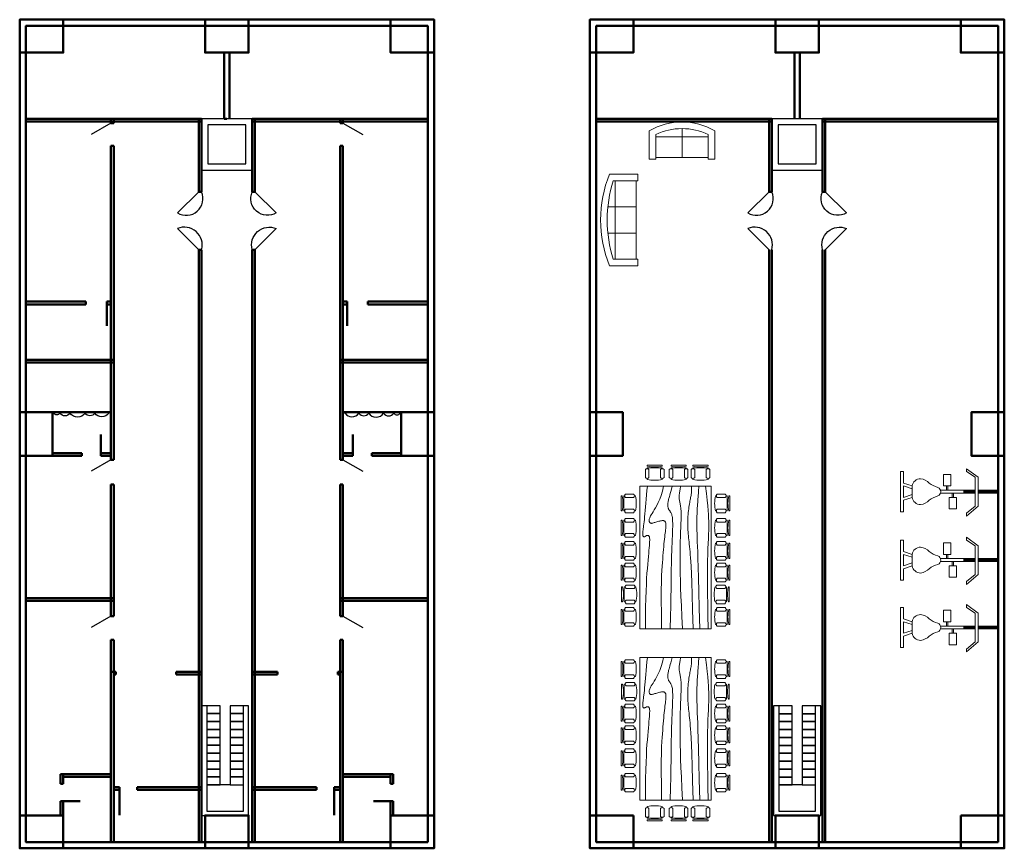
# Model space of a CAD drawing. Units: feet. Extents: x 1080 to 13444, y 870 to 7060.
# Tile 3 of 5: x 5917 to 7342, y 1047 to 2247. Entities that reach past the tile are written whole.
import ezdxf

# ---------------------------------------------------------------- set-up
doc = ezdxf.new("R2010")
doc.units = ezdxf.units.FT
for name, color, linetype, lineweight in [('A-ANNO-NPLT', 8, 'Continuous', 13), ('A-COLS', 1, 'Continuous', 50), ('A-DOOR', 4, 'Continuous', 25), ('A-FLOR-EVTR', 6, 'Continuous', 25), ('A-FLOR-STRS', 2, 'Continuous', 25), ('A-FURN', 8, 'Continuous', 18), ('A-GLAZ', 3, 'Continuous', 25), ('A-WALL', 7, 'Continuous', 50)]:
    doc.layers.add(name, color=color, linetype=linetype, lineweight=lineweight)

# ---------------------------------------------------------------- blocks, each defined once
blk = doc.blocks.new('Table - Rectangular Woodgrain 60 x 30 in.')
for p, q in [((0, 0), (0, -30)), ((60, 0), (0, 0)), ((60, -30), (60, 0)), ((0, -30), (60, -30))]:
    blk.add_line(p, q)
for points in [[(0, -2.4), (4.8155, -2.418), (9.0302, -2.4688), (12.709, -2.5477), (15.9167, -2.65), (18.7181, -2.7711), (21.1781, -2.9063), (23.3616, -3.0508), (25.3333, -3.2), (27.1477, -3.3495), (28.8172, -3.4958), (30.3437, -3.636), (31.7291, -3.7667), (32.9756, -3.8849), (34.0849, -3.9875), (35.059, -4.0714), (35.9, -4.1334), (36.6114, -4.1711), (37.2041, -4.1854), (37.6906, -4.1779), (38.0833, -4.15), (38.3948, -4.1034), (38.6375, -4.0396), (38.8239, -3.9602), (38.9666, -3.8667), (39.0764, -3.7608), (39.1573, -3.6448), (39.2116, -3.521), (39.2416, -3.3917), (39.2498, -3.2593), (39.2385, -3.1261), (39.21, -2.9944), (39.1666, -2.8667), (39.111, -2.7447), (39.0468, -2.6281), (38.978, -2.5163), (38.9083, -2.4083), (38.8418, -2.3035), (38.7823, -2.201), (38.7337, -2.1001), (38.7, -2), (38.6844, -1.9003), (38.6875, -1.8021), (38.7094, -1.707), (38.75, -1.6167), (38.8094, -1.5326), (38.8875, -1.4563), (38.9844, -1.3893), (39.1, -1.3333), (39.2351, -1.2896), (39.3937, -1.2583), (39.5804, -1.2396), (39.8, -1.2333), (40.057, -1.2396), (40.3562, -1.2583), (40.7023, -1.2896), (41.1, -1.3333), (41.5547, -1.3895), (42.0755, -1.4573), (42.6721, -1.5361), (43.3542, -1.625), (44.1316, -1.7233), (45.014, -1.8302), (46.0114, -1.9449), (47.1333, -2.0667), (48.3862, -2.1947), (49.7625, -2.3281), (51.2513, -2.4663), (52.8416, -2.6083), (54.5226, -2.7535), (56.2833, -2.9011), (58.1127, -3.0501), (60, -3.2)], [(0, -9.2), (6.5759, -9.0858), (11.9385, -9.0365), (16.2527, -9.0418), (19.6833, -9.0917), (22.3952, -9.1759), (24.5531, -9.2844), (26.322, -9.4069), (27.8666, -9.5333), (29.3241, -9.6553), (30.7203, -9.7719), (32.0532, -9.8837), (33.3208, -9.9917), (34.5213, -10.0965), (35.6526, -10.199), (36.7128, -10.2999), (37.7, -10.4), (38.6129, -10.4996), (39.4531, -10.5969), (40.223, -10.6895), (40.925, -10.775), (41.5613, -10.8512), (42.1344, -10.9156), (42.6465, -10.966), (43.1, -11), (43.4976, -11.0158), (43.8437, -11.0136), (44.143, -10.9942), (44.4, -10.9583), (44.6195, -10.9069), (44.8062, -10.8406), (44.9648, -10.7603), (45.1, -10.6667), (45.2155, -10.5598), (45.3114, -10.4365), (45.3871, -10.2929), (45.4416, -10.125), (45.4743, -9.929), (45.4844, -9.7011), (45.4709, -9.4371), (45.4333, -9.1333), (45.3716, -8.7883), (45.2896, -8.4104), (45.1919, -8.0107), (45.0833, -7.6), (44.9685, -7.1893), (44.8521, -6.7896), (44.7388, -6.4117), (44.6333, -6.0667), (44.54, -5.7628), (44.4614, -5.4979), (44.4001, -5.2675), (44.3583, -5.0667), (44.3384, -4.8909), (44.3427, -4.7354), (44.3736, -4.5956), (44.4333, -4.4667), (44.5236, -4.3453), (44.6427, -4.2333), (44.7884, -4.1339), (44.9583, -4.05), (45.1501, -3.9849), (45.3614, -3.9417), (45.59, -3.9234), (45.8333, -3.9333), (46.0915, -3.9749), (46.3734, -4.0531), (46.6906, -4.1736), (47.0542, -4.3417), (47.4756, -4.5629), (47.9661, -4.8427), (48.5372, -5.1866), (49.2, -5.6), (49.9676, -6.0844), (50.8594, -6.625), (51.8965, -7.2031), (53.1, -7.8), (54.491, -8.3969), (56.0906, -8.975), (57.9199, -9.5156), (60, -10)], [(0, -12.8), (5.1847, -12.9322), (9.6213, -13.0323), (13.3963, -13.1059), (16.5958, -13.1583), (19.3063, -13.1952), (21.614, -13.2219), (23.6054, -13.2439), (25.3666, -13.2667), (26.9728, -13.2947), (28.4531, -13.3281), (29.8256, -13.3663), (31.1083, -13.4083), (32.3191, -13.4535), (33.476, -13.501), (34.597, -13.5501), (35.7, -13.6), (36.7984, -13.6497), (37.8875, -13.6979), (38.9578, -13.743), (40, -13.7833), (41.0047, -13.8174), (41.9625, -13.8438), (42.864, -13.8607), (43.7, -13.8667), (44.4631, -13.8604), (45.1552, -13.8417), (45.7801, -13.8104), (46.3416, -13.7667), (46.8439, -13.7104), (47.2906, -13.6417), (47.6858, -13.5604), (48.0333, -13.4667), (48.3375, -13.3608), (48.6042, -13.2448), (48.8396, -13.121), (49.05, -12.9917), (49.2417, -12.8593), (49.4208, -12.7261), (49.5937, -12.5944), (49.7667, -12.4667), (49.9452, -12.3451), (50.1323, -12.2313), (50.3303, -12.1268), (50.5416, -12.0333), (50.7686, -11.9524), (51.0135, -11.8854), (51.2788, -11.8341), (51.5666, -11.8), (51.8785, -11.7843), (52.2116, -11.7865), (52.562, -11.8059), (52.926, -11.8417), (53.2998, -11.8931), (53.6795, -11.9594), (54.0614, -12.0397), (54.4416, -12.1333), (54.8223, -12.2401), (55.2293, -12.3625), (55.6942, -12.5037), (56.2489, -12.6667), (56.9251, -12.8547), (57.7545, -13.0708), (58.7689, -13.3182), (60, -13.6)], [(0, -18), (5.124, -17.7273), (9.6609, -17.5057), (13.6705, -17.3303), (17.2125, -17.1958), (20.3467, -17.0973), (23.1328, -17.0297), (25.6307, -16.9878), (27.9, -16.9667), (29.9928, -16.9617), (31.9302, -16.9703), (33.7254, -16.9907), (35.3917, -17.0208), (36.9423, -17.0588), (38.3906, -17.1026), (39.7499, -17.1503), (41.0333, -17.2), (42.2519, -17.2496), (43.4073, -17.2969), (44.4986, -17.3395), (45.525, -17.375), (46.4858, -17.4012), (47.3802, -17.4156), (48.2074, -17.416), (48.9667, -17.4), (49.6583, -17.3662), (50.2872, -17.3167), (50.8595, -17.2547), (51.3812, -17.1833), (51.8584, -17.1057), (52.2971, -17.025), (52.7034, -16.9443), (53.0833, -16.8667), (53.443, -16.7951), (53.789, -16.7313), (54.128, -16.6768), (54.4666, -16.6334), (54.8115, -16.6024), (55.1693, -16.5854), (55.5465, -16.5841), (55.95, -16.6), (56.3828, -16.6337), (56.8346, -16.6823), (57.2915, -16.7418), (57.7396, -16.8084), (58.165, -16.878), (58.5539, -16.9469), (58.8924, -17.0111), (59.1666, -17.0667), (59.3679, -17.1107), (59.5078, -17.1438), (59.6032, -17.1675), (59.6708, -17.1833), (59.7275, -17.193), (59.7901, -17.1979), (59.8753, -17.1998), (60, -17.2)], [(0, -22.4), (8.0098, -22.2501), (14.4094, -22.1011), (19.4168, -21.9535), (23.25, -21.8083), (26.1269, -21.6663), (28.2656, -21.5281), (29.884, -21.3947), (31.2, -21.2667), (32.3967, -21.1448), (33.5172, -21.0292), (34.5697, -20.9198), (35.5625, -20.8167), (36.5037, -20.7198), (37.4015, -20.6292), (38.2642, -20.5448), (39.1, -20.4667), (39.9164, -20.3951), (40.7187, -20.3313), (41.5117, -20.2768), (42.3, -20.2333), (43.0883, -20.2024), (43.8812, -20.1854), (44.6836, -20.1841), (45.5, -20.2), (46.3328, -20.234), (47.1747, -20.2844), (48.0163, -20.3488), (48.8479, -20.425), (49.66, -20.5106), (50.4429, -20.6031), (51.1872, -20.7004), (51.8833, -20.8), (52.5246, -20.8999), (53.1166, -20.9995), (53.6681, -21.0983), (54.1875, -21.1958), (54.6834, -21.2919), (55.1646, -21.3859), (55.6394, -21.4777), (56.1167, -21.5667), (56.6028, -21.6515), (57.0961, -21.7266), (57.5929, -21.7852), (58.0896, -21.8208), (58.5823, -21.8268), (59.0674, -21.7964), (59.5412, -21.723), (60, -21.6)], [(0, -25.2), (8.6355, -25.0504), (15.7026, -24.9031), (21.4049, -24.7606), (25.9458, -24.625), (29.529, -24.4988), (32.3578, -24.3844), (34.6359, -24.284), (36.5667, -24.2), (38.3213, -24.1341), (39.9417, -24.0854), (41.437, -24.0523), (42.8167, -24.0333), (44.0901, -24.0268), (45.2667, -24.0313), (46.3557, -24.0451), (47.3667, -24.0667), (48.309, -24.0947), (49.1928, -24.1287), (50.0284, -24.168), (50.826, -24.2125), (51.5959, -24.2617), (52.3483, -24.3151), (53.0935, -24.3725), (53.8417, -24.4334), (54.6009, -24.497), (55.3699, -24.561), (56.1454, -24.6226), (56.9239, -24.6792), (57.7021, -24.7279), (58.4764, -24.7662), (59.2435, -24.7911), (60, -24.8)], [(0, -28.8), (5.6867, -28.6681), (10.45, -28.5698), (14.407, -28.5012), (17.675, -28.4584), (20.3711, -28.4374), (22.6125, -28.4344), (24.5164, -28.4455), (26.2, -28.4667), (27.762, -28.4947), (29.2276, -28.5281), (30.6033, -28.5663), (31.8958, -28.6084), (33.1118, -28.6535), (34.2578, -28.7011), (35.3405, -28.7501), (36.3666, -28.8), (37.3443, -28.8497), (38.288, -28.8974), (39.2137, -28.9412), (40.1375, -28.9792), (41.0753, -29.0093), (42.0432, -29.0297), (43.0572, -29.0384), (44.1333, -29.0333), (45.2936, -29.0114), (46.5843, -28.9641), (48.0579, -28.8816), (49.7666, -28.7542), (51.7629, -28.5721), (54.0989, -28.3255), (56.8272, -28.0048), (60, -27.6)]]:
    blk.add_lwpolyline(points)
blk = doc.blocks.new('Chair - Desk')
for p, q in [((-8.5, 0), (-8.5, -1)), ((-8.5, 0), (8.5, 0)), ((8.5, 0), (8.5, -1)), ((-10.5, -5), (-10.5, -14)), ((-8.5, -3), (-8.5, -4)), ((-8.5, -3), (8.5, -3)), ((-6.5, -14), (-6.5, -5)), ((-2, -3), (-2, -1.9355)), ((2, -1.9576), (2, -3)), ((6.5, -5), (6.5, -14)), ((8.5, -3), (8.5, -4)), ((10.5, -14), (10.5, -5)), ((-8.5, -15), (-8.5, -16)), ((8.5, -15), (8.5, -16))]:
    blk.add_line(p, q)
for centre, radius, start, end in [((-8.5, -6.5), 2.5, 36.8699, 143.1301), ((0, 34.625), 36.625, 256.5803, 283.4197), ((8.5, -6.5), 2.5, 36.8699, 143.1301), ((-8.5, -12.5), 2.5, 216.8699, 323.1301), ((0, 19.625), 36.625, 256.5803, 283.4197), ((8.5, -12.5), 2.5, 216.8699, 323.1301)]:
    blk.add_arc(centre, radius, start, end)
blk = doc.blocks.new('Sofa - Roundback 7 ft.')
for p, q in [((-12.00002, -32.4421), (-12.00003, -6.5971)), ((11.99997, -32.4421), (11.99998, -6.5971)), ((-36.000027, -34), (-36.000027, -11.4696)), ((-35.999844, -13.3819), (35.9998, -13.3819)), ((35.99998, -34), (35.99998, -11.4696)), ((-36.000027, -32.4421), (35.99998, -32.4421))]:
    blk.add_line(p, q)
for points in [[(-36.000027, -34), (-42.000027, -34), (-42.000027, -8)], [(41.99998, -8), (41.99998, -34), (35.99998, -34)]]:
    blk.add_lwpolyline(points)
for centre, radius, start, end in [((0, -114.25), 114.25, 68.43141, 111.5686), ((-0.00001, -127.1968), 121.1968, 72.72033, 107.2797)]:
    blk.add_arc(centre, radius, start, end)
blk = doc.blocks.new('Sofa - Roundback Loveseat 5 ft.')
for p, q in [((0, -32.44198), (0, -5.99998)), ((-24, -33.99998), (-24, -11.46958)), ((-23.9998, -13.38178), (23.99986, -13.38178)), ((24.00004, -33.99998), (24.00004, -11.46958)), ((-24, -32.44198), (24.00004, -32.44198))]:
    blk.add_line(p, q)
for points in [[(-24, -33.99998), (-30, -33.99998), (-30, -7.99998)], [(30.00004, -7.99998), (30.00004, -33.99998), (24.00004, -33.99998)]]:
    blk.add_lwpolyline(points)
for centre, radius, start, end in [((0, -60.24998), 60.24998, 60.13715, 119.8628), ((0, -61.38438), 55.38444, 64.32083, 115.6792)]:
    blk.add_arc(centre, radius, start, end)
blk = doc.blocks.new('Exercise Bike')
for p, q in [((-0.75, 10), (-0.75, 17)), ((-0.75, 17), (0.25, 17)), ((-0.5, 17), (-0.5, 9.9929)), ((-0.25, 10), (-0.25, 17)), ((0, 17), (0, 9.9929)), ((0.25, 17), (0.25, 10)), ((-5.25, 10), (-8.25, 6)), ((-7.25, 6), (-5.25, 9)), ((-0.75, 10), (-5.25, 10)), ((-5.25, 9), (4.75, 9)), ((4.75, 10), (-0.75, 10)), ((-0.75, 5), (-0.75, 9)), ((-0.5, 8.9396), (-0.5, 5)), ((-0.25, 5), (-0.25, 9)), ((0, 8.9396), (0, 5)), ((0.25, 9), (0.25, 5)), ((8.25, 6), (4.75, 10)), ((4.75, 9), (7.25, 6)), ((-8.25, 6), (-7.25, 6)), ((-0.75, -3.0635), (-0.75, 5)), ((-0.75, 5), (0.25, 5)), ((0.25, 5), (0.25, -3.0635)), ((7.25, 6), (8.25, 6)), ((-6.25, -2), (-6.25, 0.5)), ((-2.25, 0.5), (-6.25, 0.5)), ((-2.25, -0.5), (-2.25, 0.5)), ((0.25, 1.5), (1.75, 1.5)), ((0.25, 1), (1.75, 1)), ((1.75, 2.5), (5.75, 2.5)), ((1.75, 1.5), (1.75, 2.5)), ((1.75, 1.5), (1.75, 0)), ((1.75, 0), (5.75, 0)), ((5.75, 2.5), (5.75, 0)), ((-2.25, -2), (-6.25, -2)), ((-2.25, -0.5), (-0.75, -0.5)), ((-2.25, -1), (-2.25, -0.5)), ((-2.25, -1), (-2.25, -2)), ((-0.75, -1), (-2.25, -1)), ((-2.25, -13), (-3.25, -16)), ((-2.25, -16), (-1.25, -13)), ((-2.25, -13), (1.75, -13)), ((0.75, -13), (1.75, -16)), ((1.75, -13), (2.75, -16)), ((-7.25, -16), (-7.25, -17)), ((-4.75, -16), (-7.25, -16)), ((-7.25, -17), (6.75, -17)), ((-3.25, -16), (-4.75, -16)), ((1.75, -16), (-2.25, -16)), ((6.75, -16), (2.75, -16)), ((6.75, -17), (6.75, -16))]:
    blk.add_line(p, q)
for centre, radius, start, end in [((-0.25, -4.625), 1.625, 22.61987, 157.3801), ((-9.6692, -1.9154), 8.1889, 321.6175, 345.2525), ((9.1691, -1.9154), 8.1889, 194.7476, 218.3825), ((0.1685, -10.5843), 4.9531, 133.6443, 173.2256), ((-1.7006, -10.0005), 3.0494, 179.9906, 259.6205), ((1.2006, -10.0005), 3.0494, 280.3795, 0.009389), ((-0.6686, -10.5843), 4.9531, 6.774486, 46.35562)]:
    blk.add_arc(centre, radius, start, end)
blk = doc.blocks.new('DOOR-SWING-A')
blk.add_line((30.9, 34), (0, 3.5))
blk.add_arc((12.6, 24.3), 24.3, 238.69, 23.7025)
blk = doc.blocks.new('DOOR-SWING-B')
blk.add_line((0, 30.5), (30.9, 0))
blk.add_arc((10.2, 7), 25.6, 344.0766, 113.531)

msp = doc.modelspace()

# ---------------------------------------------------------------- linework, layer by layer
at = {"layer": 'A-ANNO-NPLT'}
for p in [(6052.7, 1405), (6380.4, 1405)]:
    msp.add_point(p, dxfattribs=at)
at = {"layer": 'A-COLS'}
for points in [[(5916.5, 2246.8), (5979.5, 2246.8), (5979.5, 2199.1), (5916.5, 2199.1)], [(6185, 2246.8), (6248, 2246.8), (6248, 2199.1), (6185, 2199.1)], [(6453.5, 2246.8), (6516.5, 2246.8), (6516.5, 2199.1), (6453.5, 2199.1)], [(6742.3, 2246.8), (6805.3, 2246.8), (6805.3, 2199.1), (6742.3, 2199.1)], [(7010.8, 2246.8), (7073.8, 2246.8), (7073.8, 2199.1), (7010.8, 2199.1)], [(7279.3, 2246.8), (7342.3, 2246.8), (7342.3, 2199.1), (7279.3, 2199.1)], [(5916.5, 1615.2), (5916.5, 1678.3), (5964.2, 1678.3), (5964.2, 1615.2)], [(6516.5, 1678.3), (6516.5, 1615.2), (6468.9, 1615.2), (6468.9, 1678.3)], [(6742.3, 1615.2), (6742.3, 1678.3), (6789.9, 1678.3), (6789.9, 1615.2)], [(7342.3, 1678.3), (7342.3, 1615.2), (7294.7, 1615.2), (7294.7, 1678.3)], [(5979.5, 1094.4), (5916.5, 1094.4), (5916.5, 1046.8), (5979.5, 1046.8)], [(6248, 1046.8), (6185, 1046.8), (6185, 1094.4), (6248, 1094.4)], [(6453.5, 1094.4), (6516.5, 1094.4), (6516.5, 1046.8), (6453.5, 1046.8)], [(6805.3, 1094.4), (6742.3, 1094.4), (6742.3, 1046.8), (6805.3, 1046.8)], [(7073.8, 1046.8), (7010.8, 1046.8), (7010.8, 1094.4), (7073.8, 1094.4)], [(7279.3, 1094.4), (7342.3, 1094.4), (7342.3, 1046.8), (7279.3, 1046.8)]]:
    msp.add_lwpolyline(points, close=True, dxfattribs=at)
at = {"layer": 'A-DOOR'}
for p, q in [((6048.7, 2096.8), (6019.8, 2080.5)), ((6384.4, 2096.8), (6413.3, 2080.5)), ((6048.7, 1609.3), (6019.8, 1593)), ((6384.4, 1609.3), (6413.3, 1593)), ((6048.7, 1382.8), (6019.8, 1366.5)), ((6384.4, 1382.8), (6413.3, 1366.5))]:
    msp.add_line(p, q, dxfattribs=at)
at = {"layer": 'A-FLOR-EVTR'}
for points in [[(6179.9, 2028.8), (6253.2, 2028.8), (6253.2, 2103.4), (6179.9, 2103.4), (6179.9, 2101.1)], [(7005.7, 2028.8), (7079, 2028.8), (7079, 2103.4), (7005.7, 2103.4), (7005.7, 2101.1)], [(6189, 2037.8), (6244.1, 2037.8), (6244.1, 2094.3), (6189, 2094.3)], [(7014.7, 2037.8), (7069.9, 2037.8), (7069.9, 2094.3), (7014.7, 2094.3)]]:
    msp.add_lwpolyline(points, close=True, dxfattribs=at)
at = {"layer": 'A-FLOR-STRS'}
for points in [[(6187.5, 1253.3), (6179.9, 1253.3), (6179.9, 1094.5), (6248, 1094.5), (6248, 1253.3), (6240.4, 1253.3)], [(7015.9, 1253.1), (7008.2, 1253.1), (7008.2, 1094.4), (7076.4, 1094.4), (7076.4, 1253.1), (7068.7, 1253.1)], [(6221.3, 1138.6), (6187.5, 1138.6), (6187.5, 1100.7), (6240.4, 1100.7), (6240.4, 1138.6)], [(7049.6, 1138.5), (7015.9, 1138.5), (7015.9, 1100.6), (7068.7, 1100.6), (7068.7, 1138.5)]]:
    msp.add_lwpolyline(points, dxfattribs=at)
for points in [[(6187.5, 1253.3), (6187.5, 1241.8), (6206.6, 1241.8), (6206.6, 1253.3)], [(6187.5, 1241.8), (6187.5, 1230.3), (6206.6, 1230.3), (6206.6, 1241.8)], [(6221.3, 1253.3), (6221.3, 1241.8), (6240.4, 1241.8), (6240.4, 1253.3)], [(6221.3, 1241.8), (6221.3, 1230.3), (6240.4, 1230.3), (6240.4, 1241.8)], [(7015.9, 1253.1), (7015.9, 1241.7), (7035, 1241.7), (7035, 1253.1)], [(7015.9, 1241.7), (7015.9, 1230.2), (7035, 1230.2), (7035, 1241.7)], [(7049.6, 1253.1), (7049.6, 1241.7), (7068.7, 1241.7), (7068.7, 1253.1)], [(7049.6, 1241.7), (7049.6, 1230.2), (7068.7, 1230.2), (7068.7, 1241.7)], [(6187.5, 1230.3), (6187.5, 1218.9), (6206.6, 1218.9), (6206.6, 1230.3)], [(6221.3, 1230.3), (6221.3, 1218.9), (6240.4, 1218.9), (6240.4, 1230.3)], [(7015.9, 1230.2), (7015.9, 1218.7), (7035, 1218.7), (7035, 1230.2)], [(7049.6, 1230.2), (7049.6, 1218.7), (7068.7, 1218.7), (7068.7, 1230.2)], [(6187.5, 1218.9), (6187.5, 1207.4), (6206.6, 1207.4), (6206.6, 1218.9)], [(6221.3, 1218.9), (6221.3, 1207.4), (6240.4, 1207.4), (6240.4, 1218.9)], [(7015.9, 1218.7), (7015.9, 1207.3), (7035, 1207.3), (7035, 1218.7)], [(7049.6, 1218.7), (7049.6, 1207.3), (7068.7, 1207.3), (7068.7, 1218.7)], [(6187.5, 1207.4), (6187.5, 1195.9), (6206.6, 1195.9), (6206.6, 1207.4)], [(6221.3, 1207.4), (6221.3, 1195.9), (6240.4, 1195.9), (6240.4, 1207.4)], [(7015.9, 1207.3), (7015.9, 1195.8), (7035, 1195.8), (7035, 1207.3)], [(7049.6, 1207.3), (7049.6, 1195.8), (7068.7, 1195.8), (7068.7, 1207.3)], [(6187.5, 1195.9), (6187.5, 1184.5), (6206.6, 1184.5), (6206.6, 1195.9)], [(6187.5, 1184.5), (6187.5, 1173), (6206.6, 1173), (6206.6, 1184.5)], [(6221.3, 1195.9), (6221.3, 1184.5), (6240.4, 1184.5), (6240.4, 1195.9)], [(6221.3, 1184.5), (6221.3, 1173), (6240.4, 1173), (6240.4, 1184.5)], [(7015.9, 1195.8), (7015.9, 1184.3), (7035, 1184.3), (7035, 1195.8)], [(7015.9, 1184.3), (7015.9, 1172.9), (7035, 1172.9), (7035, 1184.3)], [(7049.6, 1195.8), (7049.6, 1184.3), (7068.7, 1184.3), (7068.7, 1195.8)], [(7049.6, 1184.3), (7049.6, 1172.9), (7068.7, 1172.9), (7068.7, 1184.3)], [(6187.5, 1173), (6187.5, 1161.5), (6206.6, 1161.5), (6206.6, 1173)], [(6221.3, 1173), (6221.3, 1161.5), (6240.4, 1161.5), (6240.4, 1173)], [(7015.9, 1172.9), (7015.9, 1161.4), (7035, 1161.4), (7035, 1172.9)], [(7049.6, 1172.9), (7049.6, 1161.4), (7068.7, 1161.4), (7068.7, 1172.9)], [(6187.5, 1161.5), (6187.5, 1150.1), (6206.6, 1150.1), (6206.6, 1161.5)], [(6221.3, 1161.5), (6221.3, 1150.1), (6240.4, 1150.1), (6240.4, 1161.5)], [(7015.9, 1161.4), (7015.9, 1149.9), (7035, 1149.9), (7035, 1161.4)], [(7049.6, 1161.4), (7049.6, 1149.9), (7068.7, 1149.9), (7068.7, 1161.4)], [(6187.5, 1150.1), (6187.5, 1138.6), (6206.6, 1138.6), (6206.6, 1150.1)], [(6221.3, 1150.1), (6221.3, 1138.6), (6240.4, 1138.6), (6240.4, 1150.1)], [(7015.9, 1149.9), (7015.9, 1138.5), (7035, 1138.5), (7035, 1149.9)], [(7049.6, 1149.9), (7049.6, 1138.5), (7068.7, 1138.5), (7068.7, 1149.9)]]:
    msp.add_lwpolyline(points, close=True, dxfattribs=at)
at = {"layer": 'A-GLAZ'}
for points in [[(6048.4, 1678.3, -0.136738), (6045.4, 1676.9, -0.520567), (6025.4, 1676.9, -0.520567), (6011.1, 1676.9, -0.520567), (5989.6, 1676.9, -0.520567), (5974.7, 1676.9, -0.520567), (5965.7, 1676.9, -0.053369), (5964.2, 1678.3, -0.053369)], [(6384.6, 1678.3, 0.136738), (6387.7, 1676.9, 0.520567), (6407.7, 1676.9, 0.520567), (6421.9, 1676.9, 0.520567), (6443.5, 1676.9, 0.520567), (6458.4, 1676.9, 0.520567), (6467.3, 1676.9, 0.053369), (6468.9, 1678.3, 0.053369)]]:
    msp.add_lwpolyline(points, format="xyb", dxfattribs=at)
at = {"layer": 'A-WALL'}
for p, q in [((6212.5, 2103.4), (6212.5, 2199.1)), ((6220.5, 2103.4), (6220.5, 2199.1)), ((7038.3, 2103.4), (7038.3, 2199.1)), ((7046.3, 2103.4), (7046.3, 2199.1)), ((6179.9, 2103.4), (5925.5, 2103.4)), ((6179.9, 2099.4), (5925.5, 2099.4)), ((6048.7, 2103.4), (6048.7, 2096.8)), ((6052.7, 2096.8), (6048.7, 2096.8)), ((6052.7, 2103.4), (6052.7, 2096.8)), ((6175.9, 2103.4), (6175.9, 1997.4)), ((6179.9, 2103.4), (6179.9, 1997.4)), ((6216.5, 2103.4), (6212.5, 2103.4)), ((6253.2, 2103.4), (6507.5, 2103.4)), ((6253.2, 2103.4), (6253.2, 1997.4)), ((6253.2, 2099.4), (6507.5, 2099.4)), ((6257.2, 2103.4), (6257.2, 1997.4)), ((6380.4, 2103.4), (6380.4, 2096.8)), ((6380.4, 2096.8), (6384.4, 2096.8)), ((6384.4, 2103.4), (6384.4, 2096.8)), ((7005.7, 2103.4), (6751.3, 2103.4)), ((7005.7, 2099.4), (6751.3, 2099.4)), ((7001.7, 2103.4), (7001.7, 1997.4)), ((7005.7, 2103.4), (7005.7, 1997.4)), ((7079, 2103.4), (7079, 1997.4)), ((7079, 2103.4), (7333.3, 2103.4)), ((7079, 2099.4), (7333.3, 2099.4)), ((7083, 2103.4), (7083, 1997.4)), ((6048.7, 2064.1), (6048.7, 1609.3)), ((6048.7, 2064.1), (6052.7, 2064.1)), ((6052.7, 2064.1), (6052.7, 1609.3)), ((6380.4, 2064.1), (6380.4, 1609.3)), ((6384.4, 2064.1), (6380.4, 2064.1)), ((6384.4, 2064.1), (6384.4, 1609.3)), ((6175.9, 1997.4), (6179.9, 1997.4)), ((6253.2, 1997.4), (6257.2, 1997.4)), ((7001.7, 1997.4), (7005.7, 1997.4)), ((7079, 1997.4), (7083, 1997.4)), ((6175.9, 1913.7), (6175.9, 1302.3)), ((6179.9, 1913.7), (6175.9, 1913.7)), ((6179.9, 1913.7), (6179.9, 1302.3)), ((6253.2, 1913.7), (6253.2, 1302.3)), ((6253.2, 1913.7), (6257.2, 1913.7)), ((6257.2, 1913.7), (6257.2, 1302.3)), ((7001.7, 1913.7), (7001.7, 1302.3)), ((7005.7, 1913.7), (7005.7, 1302.3)), ((7079, 1913.7), (7079, 1302.3)), ((7083, 1913.7), (7083, 1302.3)), ((5925.5, 1754.2), (5925.5, 1838.4)), ((5925.5, 1838.4), (6012.5, 1838.4)), ((5925.5, 1834.4), (6012.5, 1834.4)), ((6012.5, 1838.4), (6012.5, 1834.4)), ((6042.5, 1838.4), (6048.7, 1838.4)), ((6042.5, 1834.4), (6042.5, 1838.4)), ((6042.5, 1834.4), (6048.7, 1834.4)), ((6042.5, 1834.4), (6042.5, 1803.5)), ((6390.6, 1838.4), (6384.4, 1838.4)), ((6390.6, 1834.4), (6384.4, 1834.4)), ((6390.6, 1834.4), (6390.6, 1838.4)), ((6390.6, 1834.4), (6390.6, 1803.5)), ((6507.5, 1838.4), (6420.5, 1838.4)), ((6420.5, 1838.4), (6420.5, 1834.4)), ((6507.5, 1834.4), (6420.5, 1834.4)), ((6052.7, 1754.2), (5925.5, 1754.2)), ((6380.4, 1754.2), (6507.5, 1754.2)), ((6052.7, 1750.2), (5925.5, 1750.2)), ((6380.4, 1750.2), (6507.5, 1750.2)), ((5964.2, 1678.3), (6048.7, 1678.3)), ((6468.9, 1678.3), (6384.4, 1678.3)), ((6033.9, 1619.2), (6033.9, 1646)), ((6399.1, 1619.2), (6399.1, 1646)), ((5964.2, 1619.2), (6006.4, 1619.2)), ((5964.2, 1615.2), (6006.4, 1615.2)), ((6006.4, 1619.2), (6006.4, 1615.2)), ((6033.9, 1619.2), (6048.7, 1619.2)), ((6033.9, 1615.2), (6033.9, 1619.2)), ((6033.9, 1615.2), (6048.7, 1615.2)), ((6399.1, 1619.2), (6384.4, 1619.2)), ((6399.1, 1615.2), (6384.4, 1615.2)), ((6399.1, 1615.2), (6399.1, 1619.2)), ((6468.9, 1619.2), (6426.6, 1619.2)), ((6426.6, 1619.2), (6426.6, 1615.2)), ((6468.9, 1615.2), (6426.6, 1615.2)), ((6052.7, 1609.3), (6048.7, 1609.3)), ((6380.4, 1609.3), (6384.4, 1609.3)), ((6048.7, 1573.7), (6048.7, 1382.8)), ((6048.7, 1573.7), (6052.7, 1573.7)), ((6052.7, 1573.7), (6052.7, 1382.8)), ((6380.4, 1573.7), (6380.4, 1382.8)), ((6384.4, 1573.7), (6380.4, 1573.7)), ((6384.4, 1573.7), (6384.4, 1382.8)), ((6052.7, 1409), (5925.5, 1409)), ((6052.7, 1405), (5925.5, 1405)), ((6380.4, 1409), (6507.5, 1409)), ((6380.4, 1405), (6507.5, 1405)), ((6048.7, 1382.8), (6052.7, 1382.8)), ((6384.4, 1382.8), (6380.4, 1382.8)), ((6048.7, 1348.9), (6048.7, 1302.3)), ((6052.7, 1348.9), (6048.7, 1348.9)), ((6052.7, 1348.9), (6052.7, 1302.3)), ((6380.4, 1348.9), (6380.4, 1302.3)), ((6380.4, 1348.9), (6384.4, 1348.9)), ((6384.4, 1348.9), (6384.4, 1302.3)), ((6048.7, 1055.8), (6048.7, 1302.3)), ((6048.7, 1302.3), (6055.9, 1302.3)), ((6052.7, 1055.8), (6052.7, 1302.3)), ((6052.7, 1298.3), (6055.9, 1298.3)), ((6055.9, 1298.3), (6055.9, 1302.3)), ((6143.3, 1302.3), (6179.9, 1302.3)), ((6143.3, 1302.3), (6143.3, 1298.3)), ((6143.3, 1298.3), (6179.9, 1298.3)), ((6175.9, 1302.3), (6175.9, 1131.4)), ((6179.9, 1302.3), (6179.9, 1131.4)), ((6289.7, 1302.3), (6253.2, 1302.3)), ((6253.2, 1302.3), (6253.2, 1131.4)), ((6289.7, 1298.3), (6253.2, 1298.3)), ((6257.2, 1302.3), (6257.2, 1131.4)), ((6289.7, 1302.3), (6289.7, 1298.3)), ((6384.4, 1302.3), (6377.1, 1302.3)), ((6377.1, 1298.3), (6377.1, 1302.3)), ((6380.4, 1298.3), (6377.1, 1298.3)), ((6380.4, 1055.8), (6380.4, 1302.3)), ((6384.4, 1055.8), (6384.4, 1302.3)), ((7001.6, 1302.3), (7001.6, 1131.4)), ((7005.6, 1302.3), (7005.6, 1131.4)), ((7079, 1302.3), (7079, 1131.4)), ((7083, 1302.3), (7083, 1131.4)), ((5975.5, 1140.1), (5975.5, 1154.2)), ((5975.5, 1154.2), (6048.7, 1154.2)), ((5979.5, 1140.1), (5979.5, 1154.2)), ((5979.5, 1150.2), (6048.7, 1150.2)), ((6457.5, 1154.2), (6384.4, 1154.2)), ((6453.5, 1150.2), (6384.4, 1150.2)), ((6453.5, 1140.1), (6453.5, 1154.2)), ((6457.5, 1140.1), (6457.5, 1154.2)), ((5979.5, 1140.1), (5975.5, 1140.1)), ((6061.1, 1135.4), (6052.7, 1135.4)), ((6061.1, 1131.4), (6052.7, 1131.4)), ((6061.1, 1135.4), (6061.1, 1131.4)), ((6061.1, 1131.4), (6061.1, 1094.7)), ((6179.9, 1135.4), (6086.7, 1135.4)), ((6086.7, 1131.4), (6086.7, 1135.4)), ((6179.9, 1131.4), (6086.7, 1131.4)), ((6175.9, 1131.4), (6175.9, 1055.8)), ((6179.9, 1131.4), (6179.9, 1055.8)), ((6253.2, 1135.4), (6346.4, 1135.4)), ((6253.2, 1131.4), (6346.4, 1131.4)), ((6253.2, 1131.4), (6253.2, 1055.8)), ((6257.2, 1131.4), (6257.2, 1055.8)), ((6346.4, 1131.4), (6346.4, 1135.4)), ((6371.9, 1135.4), (6380.4, 1135.4)), ((6371.9, 1135.4), (6371.9, 1131.4)), ((6371.9, 1131.4), (6380.4, 1131.4)), ((6371.9, 1131.4), (6371.9, 1094.7)), ((6453.5, 1140.1), (6457.5, 1140.1)), ((7001.6, 1131.4), (7001.6, 1055.8)), ((7005.6, 1131.4), (7005.6, 1055.8)), ((7079, 1131.4), (7079, 1055.8)), ((7083, 1131.4), (7083, 1055.8)), ((5975.5, 1094.4), (5975.5, 1115)), ((5975.5, 1115), (5979.5, 1115)), ((5979.5, 1094.4), (5979.5, 1115)), ((5979.5, 1115), (6004.1, 1115)), ((6453.5, 1115), (6428.9, 1115)), ((6453.5, 1094.4), (6453.5, 1115)), ((6457.5, 1115), (6453.5, 1115)), ((6457.5, 1094.4), (6457.5, 1115))]:
    msp.add_line(p, q, dxfattribs=at)
for points in [[(6516.5, 1046.8), (5916.5, 1046.8), (5916.5, 2246.8), (6516.5, 2246.8)], [(7342.3, 1046.8), (6742.3, 1046.8), (6742.3, 2246.8), (7342.3, 2246.8)], [(6507.5, 1055.8), (5925.5, 1055.8), (5925.5, 2237.8), (6507.5, 2237.8)], [(7333.3, 1055.8), (6751.3, 1055.8), (6751.3, 2237.8), (7333.3, 2237.8)]]:
    msp.add_lwpolyline(points, close=True, dxfattribs=at)

# ---------------------------------------------------------------- block references
at = {"layer": 'A-DOOR'}
for name, p in [('DOOR-SWING-A', (6145, 1963.4)), ('DOOR-SWING-A', (6970.8, 1963.4)), ('DOOR-SWING-B', (6145, 1913.7)), ('DOOR-SWING-B', (6970.8, 1913.7))]:
    msp.add_blockref(name, p, dxfattribs=at)
at = {"layer": 'A-DOOR', "extrusion": (0, 0, -1), "zscale": -1, "rotation": 359.9998145993619}
for name, p in [('DOOR-SWING-A', (-6288.1, 1963.4)), ('DOOR-SWING-A', (-7113.9, 1963.4)), ('DOOR-SWING-B', (-6288.1, 1913.7)), ('DOOR-SWING-B', (-7113.9, 1913.7))]:
    msp.add_blockref(name, p, dxfattribs=at)
at = {"layer": 'A-FURN'}
for name, p, xscale, yscale, zscale in [('Sofa - Roundback Loveseat 5 ft.', (6875.6, 2098.5), 1.580491614545987, 1.580491614545987, 1.580491614545987), ('Chair - Desk', (6836.1, 1601.6), -1.285231871389242, 1.285231871389242, 1.285231871389242), ('Chair - Desk', (6870.7, 1601.6), -1.285231871389242, 1.285231871389242, 1.285231871389242), ('Chair - Desk', (6902.4, 1601.6), -1.285231871389242, 1.285231871389242, 1.285231871389242)]:
    msp.add_blockref(name, p, dxfattribs=dict(at, xscale=xscale, yscale=yscale, zscale=zscale))
for name, p, xscale, yscale, zscale, rotation in [('Sofa - Roundback 7 ft.', (6757.8, 1956.7), 1.580491614545987, 1.580491614545987, 1.580491614545987, 90), ('Exercise Bike', (7262.7, 1562.2), 4.15363147050826, 4.15363147050826, 4.15363147050826, 270), ('Table - Rectangular Woodgrain 60 x 30 in.', (6814.4, 1364.7), 3.443290635330402, 3.443290635330402, 3.443290635330402, 90), ('Chair - Desk', (6787.5, 1546.3), -1.285231871389242, 1.285231871389242, 1.285231871389242, 90), ('Chair - Desk', (6944.7, 1546.3), 1.285231871389242, 1.285231871389242, 1.285231871389242, 270), ('Chair - Desk', (6787.5, 1510.9), -1.285231871389242, 1.285231871389242, 1.285231871389242, 90), ('Chair - Desk', (6944.7, 1510.9), 1.285231871389242, 1.285231871389242, 1.285231871389242, 270), ('Exercise Bike', (7262.7, 1463.1), 4.15363147050826, 4.15363147050826, 4.15363147050826, 270), ('Chair - Desk', (6787.5, 1477.6), -1.285231871389242, 1.285231871389242, 1.285231871389242, 90), ('Chair - Desk', (6944.7, 1477.6), 1.285231871389242, 1.285231871389242, 1.285231871389242, 270), ('Chair - Desk', (6787.5, 1446.1), -1.285231871389242, 1.285231871389242, 1.285231871389242, 90), ('Chair - Desk', (6944.7, 1446.1), 1.285231871389242, 1.285231871389242, 1.285231871389242, 270), ('Chair - Desk', (6788.2, 1414.5), -1.285231871389242, 1.285231871389242, 1.285231871389242, 90), ('Chair - Desk', (6944, 1414.5), 1.285231871389242, 1.285231871389242, 1.285231871389242, 270), ('Exercise Bike', (7262.7, 1365.5), 4.15363147050826, 4.15363147050826, 4.15363147050826, 270), ('Chair - Desk', (6787.5, 1381.8), -1.285231871389242, 1.285231871389242, 1.285231871389242, 90), ('Chair - Desk', (6944.7, 1381.8), 1.285231871389242, 1.285231871389242, 1.285231871389242, 270), ('Chair - Desk', (6787.5, 1306.3), 1.285231871389242, 1.285231871389242, 1.285231871389242, 90), ('Table - Rectangular Woodgrain 60 x 30 in.', (6814.4, 1116.7), 3.443290635330402, 3.443290635330402, 3.443290635330402, 90), ('Chair - Desk', (6944.7, 1306.3), -1.285231871389242, 1.285231871389242, 1.285231871389242, 270), ('Chair - Desk', (6788.2, 1273.6), 1.285231871389242, 1.285231871389242, 1.285231871389242, 90), ('Chair - Desk', (6944, 1273.6), -1.285231871389242, 1.285231871389242, 1.285231871389242, 270), ('Chair - Desk', (6787.5, 1241.9), 1.285231871389242, 1.285231871389242, 1.285231871389242, 90), ('Chair - Desk', (6944.7, 1241.9), -1.285231871389242, 1.285231871389242, 1.285231871389242, 270), ('Chair - Desk', (6787.5, 1210.5), 1.285231871389242, 1.285231871389242, 1.285231871389242, 90), ('Chair - Desk', (6944.7, 1210.5), -1.285231871389242, 1.285231871389242, 1.285231871389242, 270), ('Chair - Desk', (6787.5, 1177.2), 1.285231871389242, 1.285231871389242, 1.285231871389242, 90), ('Chair - Desk', (6944.7, 1177.2), -1.285231871389242, 1.285231871389242, 1.285231871389242, 270), ('Chair - Desk', (6787.5, 1141.8), 1.285231871389242, 1.285231871389242, 1.285231871389242, 90), ('Chair - Desk', (6944.7, 1141.8), -1.285231871389242, 1.285231871389242, 1.285231871389242, 270), ('Chair - Desk', (6836.1, 1086.5), 1.285231871389242, 1.285231871389242, 1.285231871389242, 180), ('Chair - Desk', (6870.7, 1086.5), 1.285231871389242, 1.285231871389242, 1.285231871389242, 180), ('Chair - Desk', (6902.4, 1086.5), 1.285231871389242, 1.285231871389242, 1.285231871389242, 180)]:
    msp.add_blockref(name, p, dxfattribs=dict(at, xscale=xscale, yscale=yscale, zscale=zscale, rotation=rotation))

doc.saveas('drawing.dxf')
